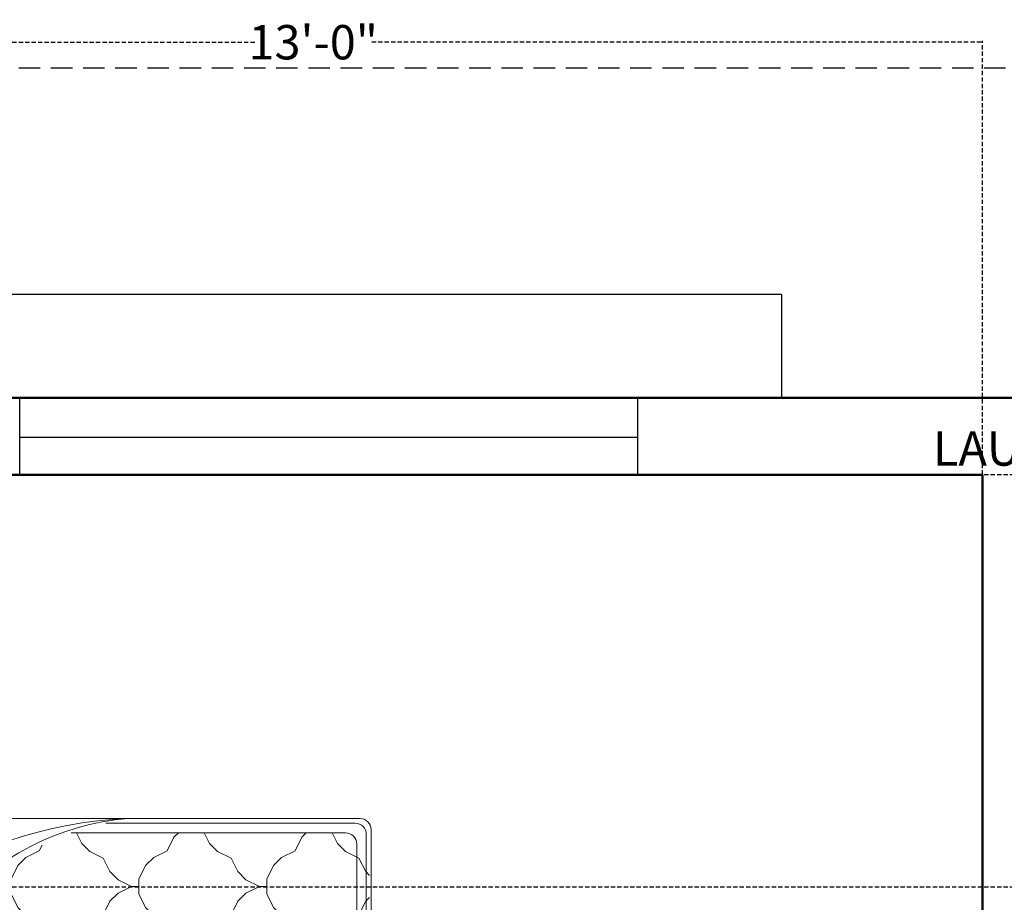
# Model space of a CAD drawing. Units: inches. Extents: x 513 to 1142, y 396 to 927.
# Tile 9 of 31: x 628 to 743, y 820 to 923. Entities that reach past the tile are written whole.
import ezdxf

# ---------------------------------------------------------------- set-up
doc = ezdxf.new("R2010")
doc.units = ezdxf.units.IN
doc.header["$MEASUREMENT"] = 0
doc.linetypes.add('DASHED', pattern=[0.75, 0.5, -0.25])
for name, color, linetype, lineweight in [('A-ANNO-DIMS', 2, 'DASHED', 18), ('A-WALL', 7, 'Continuous', 50), ('furniture', 92, 'Continuous', 18), ('windows', 172, 'Continuous', 25)]:
    doc.layers.add(name, color=color, linetype=linetype, lineweight=lineweight)
doc.styles.get("Standard").update_dxf_attribs({"font": 'arial.ttf'})
doc.dimstyles.get("Standard").update_dxf_attribs({"dimtxt": 4, "dimasz": 0.18, "dimexe": 0.18, "dimexo": 0.0625, "dimgap": 0.09, "dimtad": 0, "dimtih": 1, "dimtoh": 1, "dimdec": 0, "dimrnd": 6, "dimzin": 0, "dimdsep": 46, "dimlunit": 3, "dimtxsty": 'Standard', "dimcen": 0.09, "dimadec": 0, "dimazin": 0, "dimtfac": 1, "dimtdec": 0, "dimtofl": 0, "dimtmove": 0, "dimatfit": 3, "dimfxl": 1, "dimtolj": 1, "dimtzin": 0, "dimarcsym": 0})

# ---------------------------------------------------------------- blocks, each defined once
blk = doc.blocks.new('A$C029D5C69')
for p, q in [((0.4164, 2.0693), (0.4164, 2.0066)), ((2.2315, 2.0693), (0.4164, 2.0693)), ((2.2315, 2.0066), (2.2315, 2.0693)), ((0, 1.606), (0, 2.0066)), ((0, 2.0066), (0.505, 2.0066)), ((0.0151, 1.6211), (0.0151, 1.9915)), ((0.0151, 1.9915), (0.4899, 1.9915)), ((0.4164, 2.0066), (2.2315, 2.0066)), ((0.4899, 1.9915), (0.4899, 1.6211)), ((0.505, 2.0066), (0.505, 1.606)), ((0.5252, 0.0351), (0.5252, 2.0066)), ((0.5403, 0.0502), (0.5403, 2.0066)), ((0.5706, 0.0805), (0.5706, 2.0066)), ((0.6869, 1.966), (0.6666, 2.0066)), ((0.7072, 2.0066), (0.6869, 1.966)), ((1.0902, 1.966), (1.0699, 2.0066)), ((1.1106, 2.0066), (1.0902, 1.966)), ((2.1114, 2.0087), (2.1114, 0.0351)), ((2.6479, 2.0066), (2.1429, 2.0066)), ((2.1429, 2.0066), (2.1429, 1.606)), ((2.6328, 1.9915), (2.158, 1.9915)), ((2.158, 1.9915), (2.158, 1.6211)), ((2.6328, 1.6211), (2.6328, 1.9915)), ((2.6479, 1.606), (2.6479, 2.0066)), ((0.2689, 1.9609), (0.2689, 1.6764)), ((0.6869, 1.9425), (0.6869, 1.966)), ((0.6869, 1.9425), (0.6869, 1.966)), ((1.0902, 1.9425), (1.0902, 1.966)), ((1.0902, 1.9425), (1.0902, 1.966)), ((1.8954, 1.9865), (1.3081, 1.9865)), ((1.8954, 1.9713), (1.3339, 1.9713)), ((1.3849, 1.9713), (1.3656, 1.952)), ((1.3945, 1.9713), (1.3714, 1.9483)), ((1.4249, 1.945), (1.3986, 1.9713)), ((1.4288, 1.9507), (1.4081, 1.9713)), ((1.487, 1.9713), (1.4664, 1.9507)), ((1.4966, 1.9713), (1.4703, 1.945)), ((1.527, 1.945), (1.5007, 1.9713)), ((1.5309, 1.9507), (1.5102, 1.9713)), ((1.5891, 1.9713), (1.5685, 1.9507)), ((1.5987, 1.9713), (1.5724, 1.945)), ((1.6291, 1.945), (1.6028, 1.9713)), ((1.633, 1.9507), (1.6123, 1.9713)), ((1.6912, 1.9713), (1.6706, 1.9507)), ((1.7008, 1.9713), (1.6745, 1.945)), ((1.7312, 1.945), (1.7049, 1.9713)), ((1.7351, 1.9507), (1.7144, 1.9713)), ((1.7933, 1.9713), (1.7727, 1.9507)), ((1.8029, 1.9713), (1.7766, 1.945)), ((1.8333, 1.945), (1.807, 1.9713)), ((1.8372, 1.9507), (1.8165, 1.9713)), ((1.8954, 1.9713), (1.8748, 1.9507)), ((1.9043, 1.9707), (1.8787, 1.945)), ((1.9354, 1.945), (1.9114, 1.969)), ((2.379, 1.9609), (2.379, 1.6764)), ((0.6634, 1.9425), (0.621, 1.9213)), ((0.6634, 1.9425), (0.621, 1.9213)), ((0.6869, 1.9425), (0.6634, 1.9425)), ((0.6869, 1.9425), (0.7104, 1.9425)), ((0.7528, 1.9213), (0.7104, 1.9425)), ((0.7528, 1.9213), (0.7104, 1.9425)), ((1.0668, 1.9425), (1.0244, 1.9213)), ((1.0668, 1.9425), (1.0244, 1.9213)), ((1.0902, 1.9425), (1.0668, 1.9425)), ((1.0902, 1.9425), (1.1137, 1.9425)), ((1.1561, 1.9213), (1.1137, 1.9425)), ((1.1561, 1.9213), (1.1137, 1.9425)), ((1.4249, 1.945), (1.4059, 1.926)), ((1.4288, 1.9394), (1.4116, 1.9222)), ((1.4476, 1.9507), (1.4288, 1.9507)), ((1.4288, 1.9393), (1.4476, 1.9393)), ((1.4476, 1.9507), (1.4664, 1.9507)), ((1.4664, 1.9393), (1.4476, 1.9393)), ((1.493, 1.9128), (1.4664, 1.9394)), ((1.4986, 1.9167), (1.4703, 1.945)), ((1.527, 1.945), (1.4986, 1.9167)), ((1.5309, 1.9394), (1.5043, 1.9128)), ((1.5497, 1.9507), (1.5309, 1.9507)), ((1.5309, 1.9393), (1.5497, 1.9393)), ((1.5497, 1.9507), (1.5685, 1.9507)), ((1.5685, 1.9393), (1.5497, 1.9393)), ((1.595, 1.9128), (1.5685, 1.9394)), ((1.6007, 1.9167), (1.5724, 1.945)), ((1.6291, 1.945), (1.6007, 1.9167)), ((1.633, 1.9394), (1.6064, 1.9128)), ((1.6518, 1.9507), (1.633, 1.9507)), ((1.633, 1.9393), (1.6518, 1.9393)), ((1.6518, 1.9507), (1.6706, 1.9507)), ((1.6706, 1.9393), (1.6518, 1.9393)), ((1.6971, 1.9128), (1.6706, 1.9394)), ((1.7028, 1.9167), (1.6745, 1.945)), ((1.7312, 1.945), (1.7028, 1.9167)), ((1.7351, 1.9394), (1.7085, 1.9128)), ((1.7539, 1.9507), (1.7351, 1.9507)), ((1.7351, 1.9393), (1.7539, 1.9393)), ((1.7539, 1.9507), (1.7727, 1.9507)), ((1.7727, 1.9393), (1.7539, 1.9393)), ((1.7992, 1.9128), (1.7727, 1.9394)), ((1.8049, 1.9167), (1.7766, 1.945)), ((1.8333, 1.945), (1.8049, 1.9167)), ((1.8372, 1.9394), (1.8106, 1.9128)), ((1.856, 1.9507), (1.8372, 1.9507)), ((1.8372, 1.9393), (1.856, 1.9393)), ((1.856, 1.9507), (1.8748, 1.9507)), ((1.8748, 1.9393), (1.856, 1.9393)), ((1.9013, 1.9128), (1.8748, 1.9394)), ((1.907, 1.9167), (1.8787, 1.945)), ((1.9354, 1.945), (1.907, 1.9167)), ((1.9393, 1.9394), (1.9127, 1.9128)), ((1.9393, 1.9393), (1.9404, 1.9393)), ((1.9414, 1.688), (1.9414, 1.931)), ((1.9565, 1.688), (1.9565, 1.931)), ((0.5955, 1.8958), (0.5743, 1.8534)), ((0.621, 1.9213), (0.5955, 1.8958)), ((0.7783, 1.8958), (0.7528, 1.9213)), ((0.7995, 1.8534), (0.7783, 1.8958)), ((0.9989, 1.8958), (0.9777, 1.8534)), ((1.0243, 1.9213), (0.9988, 1.8958)), ((1.1816, 1.8958), (1.1561, 1.9213)), ((1.2028, 1.8534), (1.1816, 1.8958)), ((1.493, 1.8752), (1.493, 1.9128)), ((1.5043, 1.8752), (1.5043, 1.9128)), ((1.595, 1.8752), (1.595, 1.9128)), ((1.6064, 1.8752), (1.6064, 1.9128)), ((1.6971, 1.8752), (1.6971, 1.9128)), ((1.7085, 1.8752), (1.7085, 1.9128)), ((1.7992, 1.8752), (1.7992, 1.9128)), ((1.8106, 1.8752), (1.8106, 1.9128)), ((1.9013, 1.8752), (1.9013, 1.9128)), ((1.9127, 1.8752), (1.9127, 1.9128)), ((1.493, 1.8752), (1.4867, 1.869)), ((1.4986, 1.8713), (1.4922, 1.8648)), ((1.527, 1.8429), (1.4986, 1.8713)), ((1.5309, 1.8486), (1.5043, 1.8752)), ((1.595, 1.8752), (1.5685, 1.8486)), ((1.6007, 1.8713), (1.5724, 1.8429)), ((1.6291, 1.8429), (1.6007, 1.8713)), ((1.633, 1.8486), (1.6064, 1.8752)), ((1.6971, 1.8752), (1.6706, 1.8486)), ((1.7028, 1.8713), (1.6745, 1.8429)), ((1.7312, 1.8429), (1.7028, 1.8713)), ((1.7351, 1.8486), (1.7085, 1.8752)), ((1.7992, 1.8752), (1.7727, 1.8486)), ((1.8049, 1.8713), (1.7766, 1.8429)), ((1.8333, 1.8429), (1.8049, 1.8713)), ((1.8372, 1.8486), (1.8106, 1.8752)), ((1.9013, 1.8752), (1.8748, 1.8486)), ((1.907, 1.8713), (1.8787, 1.8429)), ((1.9354, 1.8429), (1.907, 1.8713)), ((1.9393, 1.8486), (1.9127, 1.8752)), ((0.5743, 1.8534), (0.5706, 1.8515)), ((0.5743, 1.8534), (0.5706, 1.8515)), ((0.8419, 1.8322), (0.7995, 1.8534)), ((0.8419, 1.8322), (0.7995, 1.8534)), ((0.9777, 1.8534), (0.9353, 1.8322)), ((0.9777, 1.8534), (0.9353, 1.8322)), ((1.2452, 1.8322), (1.2028, 1.8534)), ((1.2452, 1.8322), (1.2028, 1.8534)), ((1.527, 1.8429), (1.5242, 1.8401)), ((1.5309, 1.8373), (1.5295, 1.8359)), ((1.5497, 1.8486), (1.5309, 1.8486)), ((1.5309, 1.8373), (1.5497, 1.8373)), ((1.5497, 1.8486), (1.5685, 1.8486)), ((1.5685, 1.8373), (1.5497, 1.8373)), ((1.595, 1.8107), (1.5685, 1.8373)), ((1.6007, 1.8146), (1.5724, 1.8429)), ((1.6291, 1.8429), (1.6007, 1.8146)), ((1.633, 1.8373), (1.6064, 1.8107)), ((1.6518, 1.8486), (1.633, 1.8486)), ((1.633, 1.8373), (1.6518, 1.8373)), ((1.6518, 1.8486), (1.6706, 1.8486)), ((1.6706, 1.8373), (1.6518, 1.8373)), ((1.6971, 1.8107), (1.6706, 1.8373)), ((1.7028, 1.8146), (1.6745, 1.8429)), ((1.7312, 1.8429), (1.7028, 1.8146)), ((1.7351, 1.8373), (1.7085, 1.8107)), ((1.7539, 1.8486), (1.7351, 1.8486)), ((1.7351, 1.8373), (1.7539, 1.8373)), ((1.7539, 1.8486), (1.7727, 1.8486)), ((1.7727, 1.8373), (1.7539, 1.8373)), ((1.7992, 1.8107), (1.7727, 1.8373)), ((1.8049, 1.8146), (1.7766, 1.8429)), ((1.8333, 1.8429), (1.8049, 1.8146)), ((1.8372, 1.8373), (1.8106, 1.8107)), ((1.856, 1.8486), (1.8372, 1.8486)), ((1.8372, 1.8373), (1.856, 1.8373)), ((1.856, 1.8486), (1.8748, 1.8486)), ((1.8748, 1.8373), (1.856, 1.8373)), ((1.9013, 1.8107), (1.8748, 1.8373)), ((1.907, 1.8146), (1.8787, 1.8429)), ((1.9354, 1.8429), (1.907, 1.8146)), ((1.9393, 1.8373), (1.9127, 1.8107)), ((1.9414, 1.8486), (1.9393, 1.8486)), ((1.9393, 1.8373), (1.9414, 1.8373)), ((0.1267, 1.8186), (0.4111, 1.8186)), ((0.8674, 1.8067), (0.8419, 1.8322)), ((0.8886, 1.7643), (0.8674, 1.8067)), ((0.9098, 1.8067), (0.8886, 1.7643)), ((0.9352, 1.8322), (0.9097, 1.8067)), ((1.2707, 1.8067), (1.2452, 1.8322)), ((1.2919, 1.7643), (1.2707, 1.8067)), ((1.595, 1.7806), (1.595, 1.8107)), ((1.6064, 1.7731), (1.6064, 1.8107)), ((1.6971, 1.7731), (1.6971, 1.8107)), ((1.7085, 1.7731), (1.7085, 1.8107)), ((1.7992, 1.7731), (1.7992, 1.8107)), ((1.8106, 1.7731), (1.8106, 1.8107)), ((1.9013, 1.7731), (1.9013, 1.8107)), ((1.9127, 1.7731), (1.9127, 1.8107)), ((2.2367, 1.8186), (2.5212, 1.8186)), ((1.2981, 1.7768), (1.2919, 1.7643)), ((1.633, 1.7465), (1.6064, 1.7731)), ((1.6971, 1.7731), (1.6706, 1.7465)), ((1.7351, 1.7465), (1.7085, 1.7731)), ((1.7992, 1.7731), (1.7727, 1.7465)), ((1.8372, 1.7465), (1.8106, 1.7731)), ((1.9013, 1.7731), (1.8748, 1.7465)), ((1.9393, 1.7465), (1.9127, 1.7731)), ((0.8651, 1.7408), (0.8227, 1.7196)), ((0.8651, 1.7408), (0.8227, 1.7196)), ((0.912, 1.7408), (0.8651, 1.7408)), ((0.8886, 1.7408), (0.8886, 1.7643)), ((0.9544, 1.7196), (0.912, 1.7408)), ((0.9544, 1.7196), (0.912, 1.7408)), ((1.2684, 1.7408), (1.226, 1.7196)), ((1.2684, 1.7408), (1.226, 1.7196)), ((1.2885, 1.7408), (1.2684, 1.7408)), ((1.2919, 1.7519), (1.2919, 1.7643)), ((1.6518, 1.7465), (1.633, 1.7465)), ((1.6518, 1.7465), (1.6706, 1.7465)), ((1.7028, 1.7692), (1.6745, 1.7408)), ((1.7028, 1.7125), (1.6745, 1.7408)), ((1.7312, 1.7408), (1.7028, 1.7692)), ((1.7312, 1.7408), (1.7028, 1.7125)), ((1.7539, 1.7465), (1.7351, 1.7465)), ((1.7539, 1.7465), (1.7727, 1.7465)), ((1.8049, 1.7692), (1.7766, 1.7408)), ((1.8049, 1.7125), (1.7766, 1.7408)), ((1.8333, 1.7408), (1.8049, 1.7692)), ((1.8333, 1.7408), (1.8049, 1.7125)), ((1.856, 1.7465), (1.8372, 1.7465)), ((1.856, 1.7465), (1.8748, 1.7465)), ((1.907, 1.7692), (1.8787, 1.7408)), ((1.907, 1.7125), (1.8787, 1.7408)), ((1.9354, 1.7408), (1.907, 1.7692)), ((1.9354, 1.7408), (1.907, 1.7125)), ((1.9414, 1.7465), (1.9393, 1.7465)), ((0.8227, 1.7196), (0.7972, 1.6941)), ((0.98, 1.6941), (0.9545, 1.7196)), ((1.226, 1.7196), (1.2005, 1.6941)), ((1.6443, 1.7352), (1.6518, 1.7352)), ((1.6706, 1.7352), (1.6518, 1.7352)), ((1.6971, 1.7086), (1.6706, 1.7352)), ((1.6971, 1.682), (1.6971, 1.7086)), ((1.7351, 1.7352), (1.7085, 1.7086)), ((1.7085, 1.671), (1.7085, 1.7086)), ((1.7351, 1.7352), (1.7539, 1.7352)), ((1.7727, 1.7352), (1.7539, 1.7352)), ((1.7992, 1.7086), (1.7727, 1.7352)), ((1.7992, 1.671), (1.7992, 1.7086)), ((1.8372, 1.7352), (1.8106, 1.7086)), ((1.8106, 1.671), (1.8106, 1.7086)), ((1.8372, 1.7352), (1.856, 1.7352)), ((1.8748, 1.7352), (1.856, 1.7352)), ((1.9013, 1.7086), (1.8748, 1.7352)), ((1.9013, 1.671), (1.9013, 1.7086)), ((1.9393, 1.7352), (1.9127, 1.7086)), ((1.9127, 1.671), (1.9127, 1.7086)), ((1.9393, 1.7352), (1.9414, 1.7352)), ((0.5766, 1.6941), (0.5706, 1.7002)), ((0.5978, 1.6517), (0.5766, 1.6941)), ((0.7972, 1.6941), (0.776, 1.6517)), ((1.0011, 1.6517), (0.9799, 1.6941)), ((1.2005, 1.6941), (1.1793, 1.6517)), ((2.5551, 1.6275), (2.5551, 1.696)), ((0.6402, 1.6305), (0.5978, 1.6517)), ((0.6402, 1.6305), (0.5978, 1.6517)), ((0.776, 1.6517), (0.7336, 1.6305)), ((0.776, 1.6517), (0.7336, 1.6305)), ((1.0435, 1.6305), (1.0011, 1.6517)), ((1.0435, 1.6305), (1.0011, 1.6517)), ((1.1793, 1.6517), (1.1369, 1.6305)), ((1.1793, 1.6517), (1.1369, 1.6305)), ((1.7318, 1.6477), (1.7085, 1.671)), ((1.8961, 1.6477), (1.7289, 1.6477)), ((1.7992, 1.671), (1.7759, 1.6477)), ((1.8049, 1.6671), (1.7855, 1.6477)), ((1.8244, 1.6477), (1.8049, 1.6671)), ((1.8339, 1.6477), (1.8106, 1.671)), ((1.9013, 1.671), (1.878, 1.6477)), ((1.907, 1.6671), (1.8876, 1.6477)), ((1.9202, 1.6539), (1.907, 1.6671)), ((1.926, 1.6577), (1.9127, 1.671)), ((0.4899, 1.6211), (0.0151, 1.6211)), ((0.6657, 1.605), (0.6402, 1.6305)), ((0.7336, 1.6305), (0.7081, 1.605)), ((1.0691, 1.605), (1.0436, 1.6305)), ((1.1369, 1.6305), (1.1114, 1.605)), ((1.8961, 1.6325), (1.7422, 1.6325)), ((2.158, 1.6211), (2.6328, 1.6211)), ((0.505, 1.606), (0, 1.606)), ((0.6869, 1.5626), (0.6657, 1.605)), ((0.7081, 1.605), (0.6869, 1.5626)), ((1.0902, 1.5626), (1.069, 1.605)), ((1.1114, 1.605), (1.0902, 1.5626)), ((2.1429, 1.606), (2.6479, 1.606)), ((0.6869, 1.5392), (0.6869, 1.5626)), ((0.6869, 1.5392), (0.6869, 1.5626)), ((1.0902, 1.5392), (1.0902, 1.5626)), ((1.0902, 1.5392), (1.0902, 1.5626)), ((0.6634, 1.5391), (0.621, 1.5179)), ((0.6634, 1.5391), (0.621, 1.5179)), ((0.6869, 1.5392), (0.6634, 1.5392)), ((0.6869, 1.5392), (0.7104, 1.5392)), ((0.7528, 1.5179), (0.7104, 1.5391)), ((0.7528, 1.5179), (0.7104, 1.5391)), ((1.0668, 1.5391), (1.0244, 1.5179)), ((1.0668, 1.5391), (1.0244, 1.5179)), ((1.0902, 1.5392), (1.0668, 1.5392)), ((1.0902, 1.5392), (1.1137, 1.5392)), ((1.1561, 1.5179), (1.1137, 1.5391)), ((1.1561, 1.5179), (1.1137, 1.5391)), ((1.4534, 1.5308), (1.4277, 1.5179)), ((1.4534, 1.5308), (1.4277, 1.5179)), ((0.5955, 1.4925), (0.5743, 1.4501)), ((0.621, 1.5179), (0.5955, 1.4924)), ((0.7783, 1.4924), (0.7528, 1.5179)), ((0.7995, 1.4501), (0.7783, 1.4925)), ((0.9989, 1.4925), (0.9777, 1.4501)), ((1.0243, 1.5179), (0.9988, 1.4924)), ((1.1816, 1.4924), (1.1561, 1.5179)), ((1.2028, 1.4501), (1.1816, 1.4925)), ((1.4022, 1.4925), (1.381, 1.4501)), ((1.4277, 1.5179), (1.4022, 1.4924)), ((1.6062, 1.4501), (1.5966, 1.4692)), ((0.5743, 1.45), (0.5706, 1.4481)), ((0.5743, 1.45), (0.5706, 1.4481)), ((0.8419, 1.4288), (0.7995, 1.45)), ((0.8419, 1.4288), (0.7995, 1.45)), ((0.8674, 1.4033), (0.8419, 1.4288)), ((0.9352, 1.4288), (0.9097, 1.4033)), ((0.9777, 1.45), (0.9353, 1.4288)), ((0.9777, 1.45), (0.9353, 1.4288)), ((1.2452, 1.4288), (1.2028, 1.45)), ((1.2452, 1.4288), (1.2028, 1.45)), ((1.2707, 1.4033), (1.2452, 1.4288)), ((1.3386, 1.4288), (1.3131, 1.4033)), ((1.381, 1.45), (1.3386, 1.4288)), ((1.381, 1.45), (1.3386, 1.4288)), ((1.6486, 1.4288), (1.6062, 1.45)), ((1.6486, 1.4288), (1.6062, 1.45)), ((1.6741, 1.4033), (1.6486, 1.4288)), ((0.5403, 1.4117), (0.5706, 1.4117)), ((0.8886, 1.361), (0.8674, 1.4034)), ((0.9098, 1.4034), (0.8886, 1.361)), ((1.2919, 1.361), (1.2707, 1.4034)), ((1.3131, 1.4034), (1.2919, 1.361)), ((1.6953, 1.361), (1.6741, 1.4034)), ((1.714, 1.3984), (1.6953, 1.361)), ((0.8651, 1.3374), (0.8227, 1.3162)), ((0.8651, 1.3374), (0.8227, 1.3162)), ((0.912, 1.3375), (0.8651, 1.3375)), ((0.8886, 1.3375), (0.8886, 1.3609)), ((0.9544, 1.3162), (0.912, 1.3374)), ((0.9544, 1.3162), (0.912, 1.3374)), ((1.2684, 1.3374), (1.226, 1.3162)), ((1.2684, 1.3374), (1.226, 1.3162)), ((1.3154, 1.3375), (1.2684, 1.3375)), ((1.2919, 1.3375), (1.2919, 1.3609)), ((1.3578, 1.3162), (1.3154, 1.3374)), ((1.3578, 1.3162), (1.3154, 1.3374)), ((1.6718, 1.3374), (1.6294, 1.3162)), ((1.6718, 1.3374), (1.6294, 1.3162)), ((1.7187, 1.3375), (1.6718, 1.3375)), ((1.6953, 1.3375), (1.6953, 1.3609)), ((1.7611, 1.3162), (1.7187, 1.3374)), ((1.7611, 1.3162), (1.7187, 1.3374)), ((0.8227, 1.3163), (0.7972, 1.2908)), ((0.98, 1.2908), (0.9545, 1.3163)), ((1.226, 1.3163), (1.2005, 1.2908)), ((1.3833, 1.2908), (1.3578, 1.3163)), ((1.6294, 1.3163), (1.6039, 1.2908)), ((1.7867, 1.2908), (1.7611, 1.3163)), ((0.5766, 1.2908), (0.5706, 1.2968)), ((0.5978, 1.2484), (0.5766, 1.2908)), ((0.7972, 1.2908), (0.776, 1.2484)), ((1.0011, 1.2484), (0.9799, 1.2908)), ((1.2005, 1.2908), (1.1793, 1.2484)), ((1.4045, 1.2484), (1.3833, 1.2908)), ((1.6039, 1.2908), (1.5827, 1.2484)), ((1.8078, 1.2484), (1.7866, 1.2908)), ((0.6402, 1.2271), (0.5978, 1.2483)), ((0.6402, 1.2271), (0.5978, 1.2483)), ((0.776, 1.2483), (0.7336, 1.2271)), ((0.776, 1.2483), (0.7336, 1.2271)), ((1.0435, 1.2271), (1.0011, 1.2483)), ((1.0435, 1.2271), (1.0011, 1.2483)), ((1.1793, 1.2483), (1.1369, 1.2271)), ((1.1793, 1.2483), (1.1369, 1.2271)), ((1.4469, 1.2271), (1.4045, 1.2483)), ((1.4469, 1.2271), (1.4045, 1.2483)), ((1.5827, 1.2483), (1.5403, 1.2271)), ((1.5827, 1.2483), (1.5403, 1.2271)), ((1.8502, 1.2271), (1.8078, 1.2483)), ((1.8502, 1.2271), (1.8078, 1.2483)), ((0.6657, 1.2017), (0.6402, 1.2272)), ((0.7336, 1.2272), (0.7081, 1.2017)), ((1.0691, 1.2017), (1.0436, 1.2272)), ((1.1369, 1.2272), (1.1114, 1.2017)), ((1.4724, 1.2017), (1.4469, 1.2272)), ((1.5403, 1.2272), (1.5148, 1.2017)), ((1.8758, 1.2017), (1.8503, 1.2272)), ((0.5403, 1.21), (0.5706, 1.21)), ((0.6869, 1.1593), (0.6657, 1.2017)), ((0.7081, 1.2017), (0.6869, 1.1593)), ((1.0902, 1.1593), (1.069, 1.2017)), ((1.1114, 1.2017), (1.0902, 1.1593)), ((1.4936, 1.1593), (1.4724, 1.2017)), ((1.5148, 1.2017), (1.4936, 1.1593)), ((1.8969, 1.1593), (1.8757, 1.2017)), ((1.9181, 1.2017), (1.8969, 1.1593)), ((1.9215, 1.2051), (1.9181, 1.2017)), ((0.6869, 1.1358), (0.6869, 1.1593)), ((0.6869, 1.1358), (0.6869, 1.1593)), ((1.0902, 1.1358), (1.0902, 1.1593)), ((1.0902, 1.1358), (1.0902, 1.1593)), ((1.4936, 1.1358), (1.4936, 1.1593)), ((1.4936, 1.1358), (1.4936, 1.1593)), ((1.8969, 1.1358), (1.8969, 1.1593)), ((1.8969, 1.1358), (1.8969, 1.1593)), ((0.6634, 1.1358), (0.621, 1.1146)), ((0.6634, 1.1358), (0.621, 1.1146)), ((0.6869, 1.1358), (0.6634, 1.1358)), ((0.6869, 1.1358), (0.7104, 1.1358)), ((0.7528, 1.1146), (0.7104, 1.1358)), ((0.7528, 1.1146), (0.7104, 1.1358)), ((1.0668, 1.1358), (1.0244, 1.1146)), ((1.0668, 1.1358), (1.0244, 1.1146)), ((1.0902, 1.1358), (1.0668, 1.1358)), ((1.0902, 1.1358), (1.1137, 1.1358)), ((1.1561, 1.1146), (1.1137, 1.1358)), ((1.1561, 1.1146), (1.1137, 1.1358)), ((1.4701, 1.1358), (1.4277, 1.1146)), ((1.4701, 1.1358), (1.4277, 1.1146)), ((1.4936, 1.1358), (1.4701, 1.1358)), ((1.4936, 1.1358), (1.5171, 1.1358)), ((1.5595, 1.1146), (1.5171, 1.1358)), ((1.5595, 1.1146), (1.5171, 1.1358)), ((1.8735, 1.1358), (1.8311, 1.1146)), ((1.8735, 1.1358), (1.8311, 1.1146)), ((1.8969, 1.1358), (1.8735, 1.1358)), ((1.8969, 1.1358), (1.9204, 1.1358)), ((1.9628, 1.1146), (1.9204, 1.1358)), ((1.9628, 1.1146), (1.9204, 1.1358)), ((0.5955, 1.0891), (0.5743, 1.0467)), ((0.621, 1.1146), (0.5955, 1.0891)), ((0.7783, 1.0891), (0.7528, 1.1146)), ((0.7995, 1.0467), (0.7783, 1.0891)), ((0.9989, 1.0891), (0.9777, 1.0467)), ((1.0243, 1.1146), (0.9988, 1.0891)), ((1.1816, 1.0891), (1.1561, 1.1146)), ((1.2028, 1.0467), (1.1816, 1.0891)), ((1.4022, 1.0891), (1.381, 1.0467)), ((1.4277, 1.1146), (1.4022, 1.0891)), ((1.585, 1.0891), (1.5595, 1.1146)), ((1.6062, 1.0467), (1.585, 1.0891)), ((1.8056, 1.0891), (1.7844, 1.0467)), ((1.831, 1.1146), (1.8055, 1.0891)), ((1.9883, 1.0891), (1.9628, 1.1146)), ((2.0095, 1.0467), (1.9883, 1.0891)), ((0.5743, 1.0467), (0.5706, 1.0448)), ((0.5743, 1.0467), (0.5706, 1.0448)), ((0.8419, 1.0255), (0.7995, 1.0467)), ((0.8419, 1.0255), (0.7995, 1.0467)), ((0.8674, 1), (0.8419, 1.0255)), ((0.9352, 1.0255), (0.9097, 1)), ((0.9777, 1.0467), (0.9353, 1.0255)), ((0.9777, 1.0467), (0.9353, 1.0255)), ((1.2452, 1.0255), (1.2028, 1.0467)), ((1.2452, 1.0255), (1.2028, 1.0467)), ((1.2707, 1), (1.2452, 1.0255)), ((1.3386, 1.0255), (1.3131, 1)), ((1.381, 1.0467), (1.3386, 1.0255)), ((1.381, 1.0467), (1.3386, 1.0255)), ((1.6486, 1.0255), (1.6062, 1.0467)), ((1.6486, 1.0255), (1.6062, 1.0467)), ((1.6741, 1), (1.6486, 1.0255)), ((1.7419, 1.0255), (1.7164, 1)), ((1.7844, 1.0467), (1.742, 1.0255)), ((1.7844, 1.0467), (1.742, 1.0255)), ((2.0276, 1.0376), (2.0095, 1.0467)), ((2.0276, 1.0376), (2.0095, 1.0467)), ((0.8886, 0.9576), (0.8674, 1)), ((0.9098, 1), (0.8886, 0.9576)), ((1.2919, 0.9576), (1.2707, 1)), ((1.3131, 1), (1.2919, 0.9576)), ((1.6953, 0.9576), (1.6741, 1)), ((1.7165, 1), (1.6953, 0.9576)), ((0.8651, 0.9341), (0.8227, 0.9129)), ((0.8651, 0.9341), (0.8227, 0.9129)), ((0.912, 0.9341), (0.8651, 0.9341)), ((0.8886, 0.9341), (0.8886, 0.9576)), ((0.9544, 0.9129), (0.912, 0.9341)), ((0.9544, 0.9129), (0.912, 0.9341)), ((1.2684, 0.9341), (1.226, 0.9129)), ((1.2684, 0.9341), (1.226, 0.9129)), ((1.3154, 0.9341), (1.2684, 0.9341)), ((1.2919, 0.9341), (1.2919, 0.9576)), ((1.3578, 0.9129), (1.3154, 0.9341)), ((1.3578, 0.9129), (1.3154, 0.9341)), ((1.6718, 0.9341), (1.6294, 0.9129)), ((1.6718, 0.9341), (1.6294, 0.9129)), ((1.7187, 0.9341), (1.6718, 0.9341)), ((1.6953, 0.9341), (1.6953, 0.9576)), ((1.7611, 0.9129), (1.7187, 0.9341)), ((1.7611, 0.9129), (1.7187, 0.9341)), ((2.066, 0.9457), (2.066, 0.0805)), ((0.8227, 0.9129), (0.7972, 0.8874)), ((0.98, 0.8874), (0.9545, 0.9129)), ((1.226, 0.9129), (1.2005, 0.8874)), ((1.3833, 0.8874), (1.3578, 0.9129)), ((1.6294, 0.9129), (1.6039, 0.8874)), ((1.7867, 0.8874), (1.7611, 0.9129)), ((2.0327, 0.9129), (2.0072, 0.8874)), ((2.066, 0.9295), (2.0327, 0.9129)), ((2.066, 0.9295), (2.0327, 0.9129)), ((0.5766, 0.8874), (0.5706, 0.8935)), ((0.5978, 0.845), (0.5766, 0.8874)), ((0.7972, 0.8874), (0.776, 0.845)), ((1.0011, 0.845), (0.9799, 0.8874)), ((1.2005, 0.8874), (1.1793, 0.845)), ((1.4045, 0.845), (1.3833, 0.8874)), ((1.6039, 0.8874), (1.5827, 0.845)), ((1.8078, 0.845), (1.7866, 0.8874)), ((2.0072, 0.8874), (1.986, 0.845)), ((0.6402, 0.8238), (0.5978, 0.845)), ((0.6402, 0.8238), (0.5978, 0.845)), ((0.776, 0.845), (0.7336, 0.8238)), ((0.776, 0.845), (0.7336, 0.8238)), ((1.0435, 0.8238), (1.0011, 0.845)), ((1.0435, 0.8238), (1.0011, 0.845)), ((1.1793, 0.845), (1.1369, 0.8238)), ((1.1793, 0.845), (1.1369, 0.8238)), ((1.4469, 0.8238), (1.4045, 0.845)), ((1.4469, 0.8238), (1.4045, 0.845)), ((1.5827, 0.845), (1.5403, 0.8238)), ((1.5827, 0.845), (1.5403, 0.8238)), ((1.8502, 0.8238), (1.8078, 0.845)), ((1.8502, 0.8238), (1.8078, 0.845)), ((1.986, 0.845), (1.9436, 0.8238)), ((1.986, 0.845), (1.9436, 0.8238)), ((0.6657, 0.7983), (0.6402, 0.8238)), ((0.7336, 0.8238), (0.7081, 0.7983)), ((1.0691, 0.7983), (1.0436, 0.8238)), ((1.1369, 0.8238), (1.1114, 0.7983)), ((1.4724, 0.7983), (1.4469, 0.8238)), ((1.5403, 0.8238), (1.5148, 0.7983)), ((1.8758, 0.7983), (1.8503, 0.8238)), ((1.9436, 0.8238), (1.9181, 0.7983)), ((2.0962, 0.8369), (2.0962, 0.0502)), ((0.6869, 0.7559), (0.6657, 0.7983)), ((0.7081, 0.7983), (0.6869, 0.7559)), ((1.0902, 0.7559), (1.069, 0.7983)), ((1.1114, 0.7983), (1.0902, 0.7559)), ((1.4936, 0.7559), (1.4724, 0.7983)), ((1.5148, 0.7983), (1.4936, 0.7559)), ((1.8969, 0.7559), (1.8757, 0.7983)), ((1.9181, 0.7983), (1.8969, 0.7559)), ((0.6869, 0.7325), (0.6869, 0.7559)), ((0.6869, 0.7325), (0.6869, 0.7559)), ((1.0902, 0.7325), (1.0902, 0.7559)), ((1.0902, 0.7325), (1.0902, 0.7559)), ((1.2024, 0.7028), (1.2503, 0.7507)), ((1.4936, 0.7325), (1.4936, 0.7559)), ((1.4936, 0.7325), (1.4936, 0.7559)), ((1.8969, 0.7325), (1.8969, 0.7559)), ((1.8969, 0.7325), (1.8969, 0.7559)), ((0.6634, 0.7324), (0.621, 0.7112)), ((0.6634, 0.7324), (0.621, 0.7112)), ((0.6869, 0.7325), (0.6634, 0.7325)), ((0.6869, 0.7325), (0.7104, 0.7325)), ((0.7528, 0.7112), (0.7104, 0.7324)), ((0.7528, 0.7112), (0.7104, 0.7324)), ((1.0668, 0.7324), (1.0244, 0.7112)), ((1.0668, 0.7324), (1.0244, 0.7112)), ((1.0902, 0.7325), (1.0668, 0.7325)), ((1.0902, 0.7325), (1.1137, 0.7325)), ((1.1561, 0.7112), (1.1137, 0.7324)), ((1.1561, 0.7112), (1.1137, 0.7324)), ((1.4701, 0.7324), (1.4277, 0.7112)), ((1.4701, 0.7324), (1.4277, 0.7112)), ((1.4936, 0.7325), (1.4701, 0.7325)), ((1.4936, 0.7325), (1.5171, 0.7325)), ((1.5595, 0.7112), (1.5171, 0.7324)), ((1.5595, 0.7112), (1.5171, 0.7324)), ((1.8735, 0.7324), (1.8311, 0.7112)), ((1.8735, 0.7324), (1.8311, 0.7112)), ((1.8969, 0.7325), (1.8735, 0.7325)), ((1.8969, 0.7325), (1.9204, 0.7325)), ((1.9628, 0.7112), (1.9204, 0.7324)), ((1.9628, 0.7112), (1.9204, 0.7324)), ((0.5955, 0.6858), (0.5743, 0.6434)), ((0.621, 0.7113), (0.5955, 0.6858)), ((0.7783, 0.6858), (0.7528, 0.7113)), ((0.7995, 0.6434), (0.7783, 0.6858)), ((0.9989, 0.6858), (0.9777, 0.6434)), ((1.0243, 0.7113), (0.9988, 0.6858)), ((1.1816, 0.6858), (1.1561, 0.7113)), ((1.2028, 0.6434), (1.1816, 0.6858)), ((1.4022, 0.6858), (1.381, 0.6434)), ((1.4277, 0.7113), (1.4022, 0.6858)), ((1.585, 0.6858), (1.5595, 0.7113)), ((1.6062, 0.6434), (1.585, 0.6858)), ((1.8056, 0.6858), (1.7844, 0.6434)), ((1.831, 0.7113), (1.8055, 0.6858)), ((1.9883, 0.6858), (1.9628, 0.7113)), ((2.0095, 0.6434), (1.9883, 0.6858)), ((0.5743, 0.6433), (0.5706, 0.6414)), ((0.5743, 0.6433), (0.5706, 0.6414)), ((0.8419, 0.6221), (0.7995, 0.6433)), ((0.8419, 0.6221), (0.7995, 0.6433)), ((0.8674, 0.5967), (0.8419, 0.6222)), ((0.9352, 0.6222), (0.9097, 0.5967)), ((0.9777, 0.6433), (0.9353, 0.6221)), ((0.9777, 0.6433), (0.9353, 0.6221)), ((1.2452, 0.6221), (1.2028, 0.6433)), ((1.2452, 0.6221), (1.2028, 0.6433)), ((1.2707, 0.5967), (1.2452, 0.6222)), ((1.3386, 0.6222), (1.3131, 0.5967)), ((1.381, 0.6433), (1.3386, 0.6221)), ((1.381, 0.6433), (1.3386, 0.6221)), ((1.6486, 0.6221), (1.6062, 0.6433)), ((1.6486, 0.6221), (1.6062, 0.6433)), ((1.6741, 0.5967), (1.6486, 0.6222)), ((1.7419, 0.6222), (1.7164, 0.5967)), ((1.7844, 0.6433), (1.742, 0.6221)), ((1.7844, 0.6433), (1.742, 0.6221)), ((2.0519, 0.6221), (2.0095, 0.6433)), ((2.0519, 0.6221), (2.0095, 0.6433)), ((2.066, 0.6081), (2.0519, 0.6222)), ((0.8886, 0.5543), (0.8674, 0.5967)), ((0.9098, 0.5967), (0.8886, 0.5543)), ((1.2919, 0.5543), (1.2707, 0.5967)), ((1.3131, 0.5967), (1.2919, 0.5543)), ((1.6953, 0.5543), (1.6741, 0.5967)), ((1.7165, 0.5967), (1.6953, 0.5543)), ((0.8651, 0.5308), (0.8227, 0.5096)), ((0.8651, 0.5308), (0.8227, 0.5096)), ((0.912, 0.5308), (0.8651, 0.5308)), ((0.8886, 0.5308), (0.8886, 0.5543)), ((0.9544, 0.5096), (0.912, 0.5308)), ((0.9544, 0.5096), (0.912, 0.5308)), ((1.2684, 0.5308), (1.226, 0.5096)), ((1.2684, 0.5308), (1.226, 0.5096)), ((1.3154, 0.5308), (1.2684, 0.5308)), ((1.2919, 0.5308), (1.2919, 0.5543)), ((1.3578, 0.5096), (1.3154, 0.5308)), ((1.3578, 0.5096), (1.3154, 0.5308)), ((1.6718, 0.5308), (1.6294, 0.5096)), ((1.6718, 0.5308), (1.6294, 0.5096)), ((1.7187, 0.5308), (1.6718, 0.5308)), ((1.6953, 0.5308), (1.6953, 0.5543)), ((1.7611, 0.5096), (1.7187, 0.5308)), ((1.7611, 0.5096), (1.7187, 0.5308)), ((0.8227, 0.5096), (0.7972, 0.4841)), ((0.98, 0.4841), (0.9545, 0.5096)), ((1.226, 0.5096), (1.2005, 0.4841)), ((1.3833, 0.4841), (1.3578, 0.5096)), ((1.6294, 0.5096), (1.6039, 0.4841)), ((1.7867, 0.4841), (1.7611, 0.5096)), ((2.0327, 0.5096), (2.0072, 0.4841)), ((2.066, 0.5262), (2.0327, 0.5096)), ((2.066, 0.5262), (2.0327, 0.5096)), ((0.5766, 0.4841), (0.5706, 0.4901)), ((0.5978, 0.4417), (0.5766, 0.4841)), ((0.7972, 0.4841), (0.776, 0.4417)), ((1.0011, 0.4417), (0.9799, 0.4841)), ((1.2005, 0.4841), (1.1793, 0.4417)), ((1.4045, 0.4417), (1.3833, 0.4841)), ((1.6039, 0.4841), (1.5827, 0.4417)), ((1.8078, 0.4417), (1.7866, 0.4841)), ((2.0072, 0.4841), (1.986, 0.4417)), ((0.6402, 0.4205), (0.5978, 0.4417)), ((0.6402, 0.4205), (0.5978, 0.4417)), ((0.776, 0.4417), (0.7336, 0.4205)), ((0.776, 0.4417), (0.7336, 0.4205)), ((1.0435, 0.4205), (1.0011, 0.4417)), ((1.0435, 0.4205), (1.0011, 0.4417)), ((1.1793, 0.4417), (1.1369, 0.4205)), ((1.1793, 0.4417), (1.1369, 0.4205)), ((1.4469, 0.4205), (1.4045, 0.4417)), ((1.4469, 0.4205), (1.4045, 0.4417)), ((1.5827, 0.4417), (1.5403, 0.4205)), ((1.5827, 0.4417), (1.5403, 0.4205)), ((1.8502, 0.4205), (1.8078, 0.4417)), ((1.8502, 0.4205), (1.8078, 0.4417)), ((1.986, 0.4417), (1.9436, 0.4205)), ((1.986, 0.4417), (1.9436, 0.4205)), ((0.6657, 0.395), (0.6402, 0.4205)), ((0.7336, 0.4205), (0.7081, 0.395)), ((1.0691, 0.395), (1.0436, 0.4205)), ((1.1369, 0.4205), (1.1114, 0.395)), ((1.4724, 0.395), (1.4469, 0.4205)), ((1.5403, 0.4205), (1.5148, 0.395)), ((1.8758, 0.395), (1.8503, 0.4205)), ((1.9436, 0.4205), (1.9181, 0.395)), ((0.6869, 0.3526), (0.6657, 0.395)), ((0.7081, 0.395), (0.6869, 0.3526)), ((1.0902, 0.3526), (1.069, 0.395)), ((1.1114, 0.395), (1.0902, 0.3526)), ((1.4936, 0.3526), (1.4724, 0.395)), ((1.5148, 0.395), (1.4936, 0.3526)), ((1.8969, 0.3526), (1.8757, 0.395)), ((1.9181, 0.395), (1.8969, 0.3526)), ((0.6869, 0.3291), (0.6869, 0.3526)), ((0.6869, 0.3291), (0.6869, 0.3526)), ((1.0902, 0.3291), (1.0902, 0.3526)), ((1.0902, 0.3291), (1.0902, 0.3526)), ((1.4936, 0.3291), (1.4936, 0.3526)), ((1.4936, 0.3291), (1.4936, 0.3526)), ((1.8969, 0.3291), (1.8969, 0.3526)), ((1.8969, 0.3291), (1.8969, 0.3526)), ((0.6634, 0.3291), (0.621, 0.3079)), ((0.6634, 0.3291), (0.621, 0.3079)), ((0.6869, 0.3291), (0.6634, 0.3291)), ((0.6869, 0.3291), (0.7104, 0.3291)), ((0.7528, 0.3079), (0.7104, 0.3291)), ((0.7528, 0.3079), (0.7104, 0.3291)), ((1.0668, 0.3291), (1.0244, 0.3079)), ((1.0668, 0.3291), (1.0244, 0.3079)), ((1.0902, 0.3291), (1.0668, 0.3291)), ((1.0902, 0.3291), (1.1137, 0.3291)), ((1.1561, 0.3079), (1.1137, 0.3291)), ((1.1561, 0.3079), (1.1137, 0.3291)), ((1.4701, 0.3291), (1.4277, 0.3079)), ((1.4701, 0.3291), (1.4277, 0.3079)), ((1.4936, 0.3291), (1.4701, 0.3291)), ((1.4936, 0.3291), (1.5171, 0.3291)), ((1.5595, 0.3079), (1.5171, 0.3291)), ((1.5595, 0.3079), (1.5171, 0.3291)), ((1.8735, 0.3291), (1.8311, 0.3079)), ((1.8735, 0.3291), (1.8311, 0.3079)), ((1.8969, 0.3291), (1.8735, 0.3291)), ((1.8969, 0.3291), (1.9204, 0.3291)), ((1.9628, 0.3079), (1.9204, 0.3291)), ((1.9628, 0.3079), (1.9204, 0.3291)), ((0.5955, 0.2824), (0.5743, 0.24)), ((0.621, 0.3079), (0.5955, 0.2824)), ((0.7783, 0.2824), (0.7528, 0.3079)), ((0.7995, 0.24), (0.7783, 0.2824)), ((0.9989, 0.2824), (0.9777, 0.24)), ((1.0243, 0.3079), (0.9988, 0.2824)), ((1.1816, 0.2824), (1.1561, 0.3079)), ((1.2028, 0.24), (1.1816, 0.2824)), ((1.4022, 0.2824), (1.381, 0.24)), ((1.4277, 0.3079), (1.4022, 0.2824)), ((1.585, 0.2824), (1.5595, 0.3079)), ((1.6062, 0.24), (1.585, 0.2824)), ((1.8056, 0.2824), (1.7844, 0.24)), ((1.831, 0.3079), (1.8055, 0.2824)), ((1.9883, 0.2824), (1.9628, 0.3079)), ((2.0095, 0.24), (1.9883, 0.2824)), ((0.5743, 0.24), (0.5706, 0.2381)), ((0.5743, 0.24), (0.5706, 0.2381)), ((0.8419, 0.2188), (0.7995, 0.24)), ((0.8419, 0.2188), (0.7995, 0.24)), ((0.8674, 0.1933), (0.8419, 0.2188)), ((0.9352, 0.2188), (0.9097, 0.1933)), ((0.9777, 0.24), (0.9353, 0.2188)), ((0.9777, 0.24), (0.9353, 0.2188)), ((1.2452, 0.2188), (1.2028, 0.24)), ((1.2452, 0.2188), (1.2028, 0.24)), ((1.2707, 0.1933), (1.2452, 0.2188)), ((1.3386, 0.2188), (1.3131, 0.1933)), ((1.381, 0.24), (1.3386, 0.2188)), ((1.381, 0.24), (1.3386, 0.2188)), ((1.6486, 0.2188), (1.6062, 0.24)), ((1.6486, 0.2188), (1.6062, 0.24)), ((1.6741, 0.1933), (1.6486, 0.2188)), ((1.7419, 0.2188), (1.7164, 0.1933)), ((1.7844, 0.24), (1.742, 0.2188)), ((1.7844, 0.24), (1.742, 0.2188)), ((2.0519, 0.2188), (2.0095, 0.24)), ((2.0519, 0.2188), (2.0095, 0.24)), ((2.066, 0.2047), (2.0519, 0.2188)), ((0.8886, 0.1509), (0.8674, 0.1933)), ((0.9098, 0.1933), (0.8886, 0.1509)), ((1.2919, 0.1509), (1.2707, 0.1933)), ((1.3131, 0.1933), (1.2919, 0.1509)), ((1.6953, 0.1509), (1.6741, 0.1933)), ((1.7165, 0.1933), (1.6953, 0.1509)), ((0.8651, 0.1274), (0.8227, 0.1062)), ((0.8651, 0.1274), (0.8227, 0.1062)), ((0.912, 0.1275), (0.8651, 0.1275)), ((0.8886, 0.1275), (0.8886, 0.1509)), ((0.9544, 0.1062), (0.912, 0.1274)), ((0.9544, 0.1062), (0.912, 0.1274)), ((1.2684, 0.1274), (1.226, 0.1062)), ((1.2684, 0.1274), (1.226, 0.1062)), ((1.3154, 0.1275), (1.2684, 0.1275)), ((1.2919, 0.1275), (1.2919, 0.1509)), ((1.3578, 0.1062), (1.3154, 0.1274)), ((1.3578, 0.1062), (1.3154, 0.1274)), ((1.6718, 0.1274), (1.6294, 0.1062)), ((1.6718, 0.1274), (1.6294, 0.1062)), ((1.7187, 0.1275), (1.6718, 0.1275)), ((1.6953, 0.1275), (1.6953, 0.1509)), ((1.7611, 0.1062), (1.7187, 0.1274)), ((1.7611, 0.1062), (1.7187, 0.1274)), ((0.8227, 0.1062), (0.7972, 0.0807)), ((0.98, 0.0807), (0.9545, 0.1062)), ((1.226, 0.1062), (1.2005, 0.0807)), ((1.3833, 0.0807), (1.3578, 0.1062)), ((1.6294, 0.1062), (1.6039, 0.0807)), ((1.7867, 0.0807), (1.7611, 0.1062)), ((2.0327, 0.1062), (2.0072, 0.0807)), ((2.066, 0.1228), (2.0327, 0.1062)), ((2.066, 0.1228), (2.0327, 0.1062)), ((0.5766, 0.0807), (0.5706, 0.0868)), ((0.5978, 0.0384), (0.5766, 0.0808)), ((0.7972, 0.0808), (0.776, 0.0384)), ((1.0011, 0.0384), (0.9799, 0.0808)), ((1.2005, 0.0808), (1.1793, 0.0384)), ((1.4045, 0.0384), (1.3833, 0.0808)), ((1.6039, 0.0808), (1.5827, 0.0384)), ((1.8078, 0.0384), (1.7866, 0.0808)), ((2.0072, 0.0808), (1.986, 0.0384)), ((0.6402, 0.0171), (0.5978, 0.0383)), ((0.6402, 0.0171), (0.5978, 0.0383)), ((2.0309, 0.0454), (0.6056, 0.0454)), ((0.776, 0.0383), (0.7336, 0.0171)), ((0.776, 0.0383), (0.7336, 0.0171)), ((1.0435, 0.0171), (1.0011, 0.0383)), ((1.0435, 0.0171), (1.0011, 0.0383)), ((1.1793, 0.0383), (1.1369, 0.0171)), ((1.1793, 0.0383), (1.1369, 0.0171)), ((1.4469, 0.0171), (1.4045, 0.0383)), ((1.4469, 0.0171), (1.4045, 0.0383)), ((1.5827, 0.0383), (1.5403, 0.0171)), ((1.5827, 0.0383), (1.5403, 0.0171)), ((1.8502, 0.0171), (1.8078, 0.0383)), ((1.8502, 0.0171), (1.8078, 0.0383)), ((1.986, 0.0383), (1.9436, 0.0171)), ((1.986, 0.0383), (1.9436, 0.0171)), ((2.0763, 0), (0.5603, 0)), ((2.0612, 0.0151), (0.5754, 0.0151)), ((0.6523, 0.005), (0.6402, 0.0171)), ((0.7336, 0.0171), (0.7215, 0.005)), ((1.0557, 0.005), (1.0436, 0.0171)), ((1.1369, 0.0171), (1.1248, 0.005)), ((1.459, 0.005), (1.4469, 0.0171)), ((1.5403, 0.0171), (1.5282, 0.005)), ((1.8623, 0.005), (1.8503, 0.0171)), ((1.9436, 0.0171), (1.9315, 0.005))]:
    blk.add_line(p, q)
at = {"ltscale": 0.005}
for p, q in [((0.4899, 1.6568), (0.0151, 1.9915)), ((0.0151, 1.6568), (0.4899, 1.9915)), ((2.6328, 1.6568), (2.158, 1.9915)), ((2.158, 1.6568), (2.6328, 1.9915)), ((0.0151, 1.6568), (0.4899, 1.6568)), ((2.6328, 1.6568), (2.158, 1.6568))]:
    blk.add_line(p, q, dxfattribs=at)
for centre, radius in [((0.2689, 1.8186), 0.1191), ((2.379, 1.8186), 0.1191), ((0.2689, 1.8186), 0.0711), ((2.379, 1.8186), 0.0711)]:
    blk.add_circle(centre, radius)
for centre, radius, start, end in [((0.2843, 0.0157), 0.6251, 10.2961, 13.2684), ((0.6056, 0.0805), 0.0351, 180, 270), ((2.0309, 0.0805), 0.0351, 270, 0), ((0.5603, 0.0351), 0.0351, 180, 270), ((0.5754, 0.0502), 0.0351, 180, 270), ((2.0612, 0.0502), 0.0351, 270, 0), ((2.0763, 0.0351), 0.0351, 270, 0)]:
    blk.add_arc(centre, radius, start, end)
for centre, major_axis, ratio, start_param, end_param in [((0.8506, 1.8527), (-0.4556, 0), 0.89, 2.430919, 3.53111), ((0.3667, 0.6698), (1.7398, 0.1668), 0.88072, -0.045073, 0.941433), ((1.8961, 1.931), (-0.0453, 0), 0.89, 3.141593, 4.712389), ((1.8961, 1.688), (-0.0453, 0), 0.89, 1.570796, 3.141593), ((1.0874, 0.6748), (1.021, 0.1213), 0.889348, -0.031673, 1.359628)]:
    blk.add_ellipse(centre, major_axis=major_axis, ratio=ratio, start_param=start_param, end_param=end_param)
for points, knots in [([(1.9565, 1.931), (1.9565, 1.9336), (1.9563, 1.9362), (1.9553, 1.9428), (1.9543, 1.9467), (1.9512, 1.9541), (1.9493, 1.9577), (1.9446, 1.9643), (1.942, 1.9674), (1.936, 1.9729), (1.9327, 1.9753), (1.9257, 1.9795), (1.922, 1.9813), (1.9142, 1.9841), (1.9102, 1.9851), (1.9028, 1.9862), (1.8995, 1.9865), (1.8961, 1.9865)], [3.141593, 3.141593, 3.141593, 3.141593, 3.277614, 3.277614, 3.488082, 3.488082, 3.698551, 3.698551, 3.909019, 3.909019, 4.119488, 4.119488, 4.329956, 4.329956, 4.540424, 4.540424, 4.712389, 4.712389, 4.712389, 4.712389]), ([(1.8961, 1.6325), (1.899, 1.6325), (1.9019, 1.6327), (1.9101, 1.6338), (1.9153, 1.6352), (1.9253, 1.6392), (1.93, 1.6418), (1.9385, 1.6481), (1.9423, 1.6519), (1.9481, 1.6594), (1.9503, 1.663), (1.9537, 1.6707), (1.955, 1.6747), (1.9563, 1.6818), (1.9565, 1.6849), (1.9565, 1.688)], [1.570796, 1.570796, 1.570796, 1.570796, 1.718836, 1.718836, 1.993452, 1.993452, 2.268068, 2.268068, 2.542684, 2.542684, 2.761386, 2.761386, 2.980087, 2.980087, 3.141593, 3.141593, 3.141593, 3.141593])]:
    blk.add_open_spline(points, degree=3, knots=knots)
blk = doc.blocks.new('A$C0D3A6DFA')
blk.add_blockref('A$C029D5C69', (0, 0))
blk = doc.blocks.new('*D103')
at = {"layer": 'A-ANNO-DIMS', "color": 0, "lineweight": -2, "ltscale": 5, "transparency": 16777216}
for p, q in [((575, 879.22), (575, 917.74)), ((575.18, 917.56), (828.93, 917.56)), ((1089.82, 917.56), (836.06, 917.56)), ((1090, 879.22), (1090, 917.74))]:
    blk.add_line(p, q, dxfattribs=at)
at = {"layer": 'A-ANNO-DIMS', "color": 0, "ltscale": 5, "transparency": 16777216}
for points in [[(575.18, 917.59), (575.18, 917.53), (575, 917.56)], [(1089.82, 917.59), (1089.82, 917.53), (1090, 917.56)]]:
    blk.add_solid(points, dxfattribs=at)
at = {"layer": 'Defpoints', "color": 0, "ltscale": 5, "transparency": 16777216}
for p in [(1090, 917.56), (575, 879.16), (1090, 879.16)]:
    blk.add_point(p, dxfattribs=at)
at = {"layer": 'A-ANNO-DIMS', "color": 0, "ltscale": 5, "transparency": 16777216, "insert": (832.5, 917.56), "char_height": 4, "attachment_point": 5}
blk.add_mtext("\\A1;43'", dxfattribs=at)
blk = doc.blocks.new('WIN-72IN')
blk.add_line((0, 4.45), (72, 4.45))
blk.add_lwpolyline([(72, 9), (72, 0), (0, 0), (0, 9)], close=True)
blk = doc.blocks.new('*D115')
at = {"layer": 'A-ANNO-DIMS', "color": 0, "lineweight": -2, "transparency": 16777216}
for p, q in [((812.39, 873.24), (812.21, 873.24)), ((812.39, 869.76), (812.39, 873.42)), ((835.83, 873.24), (812.57, 873.24)), ((836.01, 869.76), (836.01, 873.42))]:
    blk.add_line(p, q, dxfattribs=at)
at = {"layer": 'A-ANNO-DIMS', "color": 0, "transparency": 16777216}
for points in [[(812.57, 873.27), (812.57, 873.21), (812.39, 873.24)], [(835.83, 873.27), (835.83, 873.21), (836.01, 873.24)]]:
    blk.add_solid(points, dxfattribs=at)
at = {"layer": 'Defpoints', "color": 0, "transparency": 16777216}
for p in [(812.39, 873.24), (812.39, 869.7), (836.01, 869.7)]:
    blk.add_point(p, dxfattribs=at)
at = {"layer": 'A-ANNO-DIMS', "color": 0, "transparency": 16777216, "insert": (772.38, 873.24), "char_height": 4, "attachment_point": 5}
blk.add_mtext('\\A1;LAUNDRY UNIT 1\'-11 1/2" TYP.', dxfattribs=at)
blk = doc.blocks.new('*D135')
at = {"layer": 'A-ANNO-DIMS', "color": 0, "lineweight": -2, "transparency": 16777216}
for p, q in [((584, 870.22), (584, 920.74)), ((584.18, 920.56), (655.22, 920.56)), ((739.82, 920.56), (668.77, 920.56)), ((740, 870.22), (740, 920.74))]:
    blk.add_line(p, q, dxfattribs=at)
at = {"layer": 'A-ANNO-DIMS', "color": 0, "transparency": 16777216}
for points in [[(584.18, 920.59), (584.18, 920.53), (584, 920.56)], [(739.82, 920.59), (739.82, 920.53), (740, 920.56)]]:
    blk.add_solid(points, dxfattribs=at)
at = {"layer": 'Defpoints', "color": 0, "transparency": 16777216}
for p in [(740, 920.56), (584, 870.16), (740, 870.16)]:
    blk.add_point(p, dxfattribs=at)
at = {"layer": 'A-ANNO-DIMS', "color": 0, "transparency": 16777216, "insert": (662, 920.56), "char_height": 4, "attachment_point": 5}
blk.add_mtext('\\A1;13\'-0"', dxfattribs=at)
blk = doc.blocks.new('*D170')
at = {"layer": 'A-ANNO-DIMS', "color": 0, "lineweight": -2, "transparency": 16777216}
for p, q in [((835.93, 870.16), (533.42, 870.16)), ((533.6, 869.98), (533.6, 848.29)), ((533.6, 822.34), (533.6, 844.03)), ((835.93, 822.16), (533.42, 822.16))]:
    blk.add_line(p, q, dxfattribs=at)
at = {"layer": 'A-ANNO-DIMS', "color": 0, "transparency": 16777216}
for points in [[(533.57, 869.98), (533.63, 869.98), (533.6, 870.16)], [(533.57, 822.34), (533.63, 822.34), (533.6, 822.16)]]:
    blk.add_solid(points, dxfattribs=at)
at = {"layer": 'Defpoints', "color": 0, "transparency": 16777216}
for p in [(533.6, 870.16), (836, 870.16), (836, 822.16)]:
    blk.add_point(p, dxfattribs=at)
at = {"layer": 'A-ANNO-DIMS', "color": 0, "transparency": 16777216, "insert": (533.6, 846.16), "char_height": 4, "attachment_point": 5}
blk.add_mtext('\\A1;4\'-0"', dxfattribs=at)

msp = doc.modelspace()

# ---------------------------------------------------------------- linework, layer by layer
at = {"layer": 'A-WALL'}
for p, q in [((1090, 879.16), (575, 879.16)), ((740, 870.16), (584, 870.16)), ((740, 870.16), (740, 710.16))]:
    msp.add_line(p, q, dxfattribs=at)
at = {"layer": 'windows'}
for q in [(617.06, 891.16), (716.56, 879.16)]:
    msp.add_line((716.56, 891.16), q, dxfattribs=at)

# ---------------------------------------------------------------- block references
at = {"layer": 'furniture', "xscale": 36.93602985360944, "yscale": 36.93602985360944, "zscale": 36.93602985360944, "rotation": 90}
msp.add_blockref('A$C0D3A6DFA', (668.74, 752.17), dxfattribs=at)
at = {"layer": 'windows'}
msp.add_blockref('WIN-72IN', (627.79, 870.12), dxfattribs=at)

# ---------------------------------------------------------------- dimensions: what is measured, and where the dimension line sits
at = {"layer": 'A-ANNO-DIMS'}
dim = msp.add_linear_dim(base=(740, 920.56), p1=(584, 870.16), p2=(740, 870.16), dimstyle='Standard', override={"dimdec": 1, "dimlfac": 1, "dimrnd": 0, "dimzin": 1, "dimdsep": 46, "dimlunit": 4, "dimfrac": 2}, dxfattribs=at)
dim.commit()
dim.dimension.update_dxf_attribs({"geometry": '*D135', "text_midpoint": (662, 920.56)})
at = {"layer": 'A-ANNO-DIMS', "ltscale": 5}
dim = msp.add_linear_dim(base=(1090, 917.56), p1=(575, 879.16), p2=(1090, 879.16), dimstyle='Standard', override={"dimclrd": 0, "dimclre": 0, "dimclrt": 0}, dxfattribs=at)
dim.commit()
dim.dimension.update_dxf_attribs({"geometry": '*D103', "text_midpoint": (832.5, 917.56)})
at = {"layer": 'A-ANNO-DIMS'}
dim = msp.add_linear_dim(base=(812.39, 873.24), p1=(836.01, 869.7), p2=(812.39, 869.7), angle=180, text='LAUNDRY UNIT <> TYP.', dimstyle='Standard', override={"dimdec": 1, "dimlfac": 1, "dimrnd": 0, "dimzin": 1, "dimdsep": 46, "dimlunit": 4, "dimfrac": 2}, dxfattribs=at)
dim.commit()
dim.dimension.update_dxf_attribs({"geometry": '*D115', "text_midpoint": (772.38, 873.24)})
dim = msp.add_linear_dim(base=(533.6, 870.16), p1=(836, 822.16), p2=(836, 870.16), angle=90, dimstyle='Standard', override={"dimdec": 1, "dimlfac": 1, "dimrnd": 0, "dimzin": 1, "dimdsep": 46, "dimlunit": 4, "dimfrac": 2}, dxfattribs=at)
dim.commit()
dim.dimension.update_dxf_attribs({"geometry": '*D170', "text_midpoint": (533.6, 846.16)})

doc.saveas('drawing.dxf')
